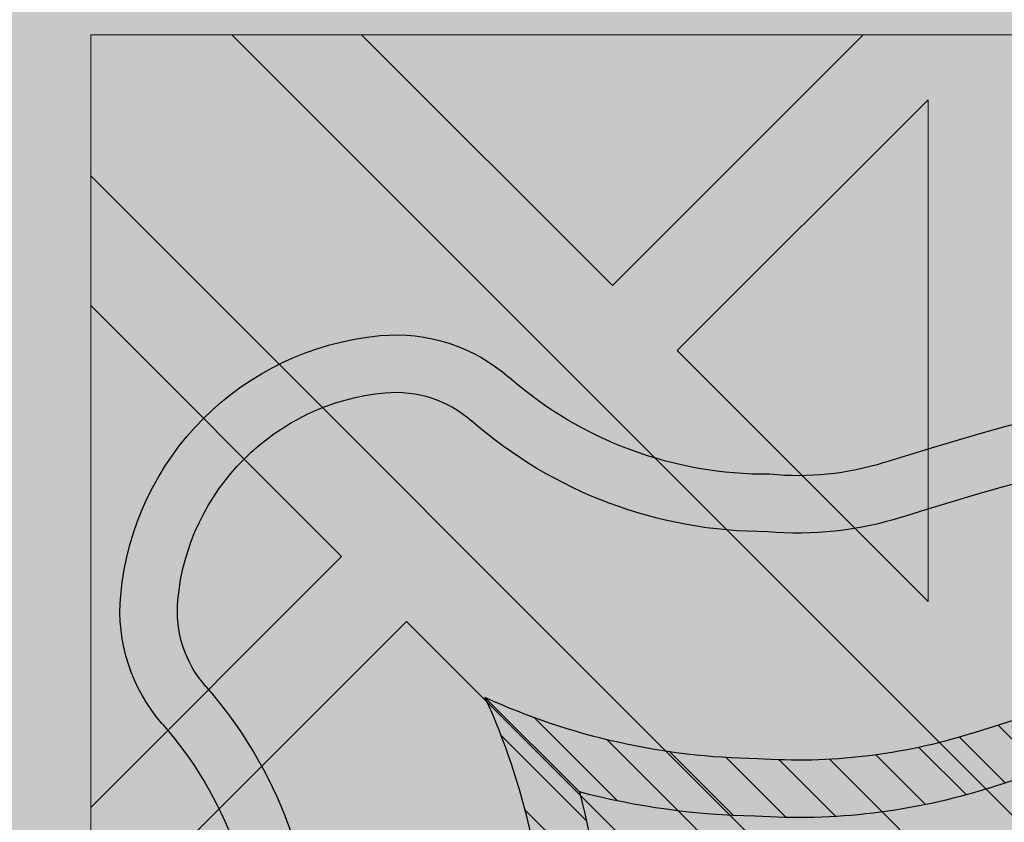
# Model space of a CAD drawing. Units: inches. Extents: x 844 to 2234, y 346 to 1084.
# Tile 81 of 93: x 1999.197 to 2001.933, y 708.742 to 710.971. Entities that reach past the tile are written whole.
import ezdxf

# ---------------------------------------------------------------- set-up
doc = ezdxf.new("R2010")
doc.units = ezdxf.units.IN
doc.header["$MEASUREMENT"] = 0
for name, color, linetype, lineweight in [('A-ANNO-DIMS', 2, 'Continuous', 18), ('furniture', 8, 'Continuous', 18), ('RA-AP-01$0$INT', 35, 'Continuous', 5)]:
    doc.layers.add(name, color=color, linetype=linetype, lineweight=lineweight)
doc.layers.add('RA-AP-01$0$FURN', color=3, linetype='Continuous')
doc.layers.add('RA-AP-01$0$WOOD', color=64, linetype='Continuous')
doc.styles.get("Standard").update_dxf_attribs({"font": 'arial.ttf'})
doc.dimstyles.get("Standard").update_dxf_attribs({"dimtxt": 6, "dimasz": 3, "dimexe": 0.18, "dimexo": 0.0625, "dimgap": 0.09, "dimtad": 0, "dimtih": 1, "dimtoh": 1, "dimdec": 1, "dimzin": 0, "dimdsep": 46, "dimlunit": 3, "dimtxsty": 'Standard', "dimblk": 'ARCHTICK', "dimcen": 0.09, "dimadec": 0, "dimazin": 0, "dimtfac": 1, "dimtdec": 1, "dimtofl": 0, "dimtmove": 0, "dimatfit": 3, "dimfxl": 1, "dimtolj": 1, "dimtzin": 0, "dimarcsym": 0})

# ---------------------------------------------------------------- blocks, each defined once
blk = doc.blocks.new('A$C18D01794')
at = {"layer": 'RA-AP-01$0$INT'}
blk.add_hatch(color=256, dxfattribs=at).paths.add_polyline_path([(4.505206456958071, -7.906712009588039), (5.305206456958072, -7.906712009588039), (5.305206456958072, -7.106712009588038), (5.255206456951893, -7.106712009588036), (5.25520645694868, -7.856712009570104), (4.555206456959269, -7.856712009588616), (4.555206456956052, -7.106712009588038), (4.505206456958073, -7.106712009588038)])
h = blk.add_hatch(color=256, dxfattribs=at)
h.paths.add_polyline_path([(4.585917135068448, -7.856712009587804), (4.614201406330596, -7.856712009587056), (4.668846067270487, -7.802067348644738), (4.723490728212344, -7.856712009584164), (4.771774999457151, -7.856712009582887), (4.826419660396886, -7.80206734864072), (4.862780050090322, -7.838427738332541), (4.844495778842715, -7.856712009580965), (4.862780050090411, -7.856712009580482), (4.905206456960182, -7.814285602707865), (4.947632863832445, -7.856712009578238), (4.965917135079675, -7.856712009577755), (4.947632863831759, -7.838427738330656), (4.983993253523576, -7.802067348637219), (5.038637914464627, -7.856712009575829), (5.08692218571208, -7.856712009574554), (5.141566846649976, -7.802067348634224), (5.196211507589851, -7.856712009571666), (5.224495778822615, -7.856712009570916), (4.905206456953975, -7.537422687702283)])
h.paths.add_polyline_path([(4.895206456956031, -7.575706958950402), (4.895206456958921, -7.684996280828174), (4.840561796018589, -7.630351619890275)], flags=16)
h.paths.add_polyline_path([(4.915206456955638, -7.575706958949956), (4.969851117895509, -7.630351619887399), (4.915206456957609, -7.684996280827732)], flags=16)
h.paths.add_polyline_path([(4.826419660395175, -7.644493755514321), (4.881064321335613, -7.699138416452331), (4.771774999456703, -7.69913841645522)], flags=16)
h.paths.add_polyline_path([(4.983993253519558, -7.644493755510815), (5.038637914460456, -7.699138416449285), (4.929348592581548, -7.69913841645126)], flags=16)
h.paths.add_polyline_path([(4.881064321336025, -7.719138416452334), (4.826419660397532, -7.773783077393256), (4.771774999457062, -7.719138416455217)], flags=16)
h.paths.add_polyline_path([(4.929348592582019, -7.71913841645126), (5.038637914460982, -7.719138416449284), (4.983993253522945, -7.773783077389749)], flags=16)
h.paths.add_polyline_path([(4.895206456960191, -7.733280552075633), (4.895206456962115, -7.806001331460164), (4.876922185715016, -7.824285602708492), (4.840561796021581, -7.787925213016675)], flags=16)
h.paths.add_polyline_path([(4.915206456958487, -7.733280552075187), (4.969851117899527, -7.787925213013798), (4.933490728206909, -7.824285602708034), (4.9152064569598, -7.806001331461736)], flags=16)
h.paths.add_polyline_path([(4.757632863832376, -7.733280552079264), (4.812277524772842, -7.787925213017304), (4.757632863834348, -7.842569873958233)], flags=16)
h.paths.add_polyline_path([(4.737632863832376, -7.73328055207979), (4.737632863834348, -7.842569873958701), (4.682988202893906, -7.787925213020692)], flags=16)
h.paths.add_polyline_path([(5.05278005008503, -7.733280552072701), (5.052780050087917, -7.842569873951664), (4.998135389146995, -7.787925213013169)], flags=16)
h.paths.add_polyline_path([(5.072780050085024, -7.733280552072333), (5.127424711025931, -7.787925213010806), (5.072780050087916, -7.842569873951244)], flags=16)
h.paths.add_polyline_path([(4.935917135072783, -7.506712009583784), (5.255206456948811, -7.826001331459767), (5.255206456948932, -7.797717060211899), (5.200561796010279, -7.743072399273238), (5.255206456949403, -7.688427738334128), (5.25520645694961, -7.640143467086677), (5.200561796009787, -7.585498806146837), (5.236922185702417, -7.549138416454212), (5.255206456949919, -7.56742268770172), (5.255206456949998, -7.549138416454178), (5.212780050078687, -7.506712009583814), (5.25520645695036, -7.464285602712145), (5.255206456950438, -7.446001331464763), (5.236922185702424, -7.464285602712779), (5.200561796009796, -7.427925213020149), (5.255206456950753, -7.373280552079203), (5.25520645695096, -7.324996280834394), (5.200561796010322, -7.270351619893748), (5.255206456951428, -7.215706958952649), (5.255206456951547, -7.187422687705071)])
h.paths.add_polyline_path([(5.042988202883395, -7.42792521302065), (5.097632863823085, -7.373280552080975), (5.097632863822622, -7.482569873959883)], flags=16)
h.paths.add_polyline_path([(5.028846067259663, -7.442067348644384), (5.083490728198774, -7.496712009583504), (4.974201406321001, -7.496712009583035)], flags=16)
h.paths.add_polyline_path([(5.117632863823087, -7.37328055208089), (5.172277524762331, -7.42792521302015), (5.11763286382262, -7.482569873959851)], flags=16)
h.paths.add_polyline_path([(5.08349072819877, -7.516712009582191), (5.028846067259652, -7.571356670521302), (4.974201406320998, -7.516712009582638)], flags=16)
h.paths.add_polyline_path([(5.131774999446817, -7.35913841645716), (5.186419660386065, -7.413783077396415), (5.241064321325782, -7.359138416456712)], flags=17)
h.paths.add_polyline_path([(5.131774999446228, -7.496712009583703), (5.186419660386065, -7.442067348643883), (5.222780050079488, -7.478427738337313), (5.204495778832781, -7.496712009584014)], flags=16)
h.paths.add_polyline_path([(5.097632863822613, -7.530854145205813), (5.097632863823061, -7.640143467084723), (5.042988202883383, -7.585498806145032)], flags=16)
h.paths.add_polyline_path([(5.131774999446899, -7.339138416457162), (5.241064321325809, -7.339138416456712), (5.186419660386591, -7.284493755517479)], flags=17)
h.paths.add_polyline_path([(5.131774999446226, -7.516712009581999), (5.204495778830767, -7.516712009581702), (5.22278005007868, -7.534996280829206), (5.186419660386049, -7.571356670521828)], flags=16)
h.paths.add_polyline_path([(5.11763286382262, -7.530854145205852), (5.17227752476232, -7.585498806145562), (5.117632863823064, -7.64014346708481)], flags=16)
h.paths.add_polyline_path([(5.186419660386069, -7.599640941770585), (5.241064321325754, -7.654285602710281), (5.131774999446791, -7.654285602709814)], flags=16)
h.paths.add_polyline_path([(5.131774999446872, -7.674285602709813), (5.24106432132578, -7.674285602710282), (5.186419660386554, -7.728930263649504)], flags=16)
h.paths.add_polyline_path([(5.255206456951811, -7.126001331467467), (5.255206456951895, -7.106712009588038), (4.555206456956052, -7.106712009588038), (4.555206456956136, -7.12600133146746), (4.905206456953973, -7.476001331465289)])
h.paths.add_polyline_path([(4.983993253513404, -7.368930263651977), (4.92934859257295, -7.314285602713969), (5.03863791445186, -7.314285602711063)], flags=16)
h.paths.add_polyline_path([(4.969851117889988, -7.383072399276016), (4.915206456952556, -7.437717060215906), (4.915206456949648, -7.328427738338133)], flags=16)
h.paths.add_polyline_path([(4.929348592572535, -7.294285602713971), (4.983993253511019, -7.239640941773039), (5.038637914451496, -7.294285602711065)], flags=16)
h.paths.add_polyline_path([(5.052780050074912, -7.280143467087016), (4.998135389134438, -7.225498806148989), (5.052780050072919, -7.170854145208052)], flags=16)
h.paths.add_polyline_path([(5.07278005007491, -7.280143467086489), (5.072780050072918, -7.170854145207579), (5.127424711013374, -7.225498806145578)], flags=16)
h.paths.add_polyline_path([(4.89520645695295, -7.437717060216355), (4.840561796013067, -7.383072399278919), (4.895206456950961, -7.328427738338582)], flags=16)
h.paths.add_polyline_path([(4.915206456948365, -7.280143467090674), (4.915206456946434, -7.207422687704125), (4.933490728192729, -7.18913841645701), (4.969851117886972, -7.225498806149623)], flags=16)
h.paths.add_polyline_path([(4.881064321327021, -7.314285602715054), (4.82641966038902, -7.368930263655506), (4.771774999448108, -7.314285602717047)], flags=16)
h.paths.add_polyline_path([(4.895206456950073, -7.280143467091125), (4.840561796009022, -7.225498806152518), (4.876922185700835, -7.18913841645908), (4.895206456948749, -7.207422687706589)], flags=16)
h.paths.add_polyline_path([(4.983993253510392, -7.211356670525576), (4.947632863816944, -7.174996280833758), (4.965917135064043, -7.156712009585847), (5.038637914448995, -7.156712009584522)], flags=16)
h.paths.add_polyline_path([(4.881064321326543, -7.294285602715056), (4.771774999447578, -7.294285602717046), (4.826419660385607, -7.239640941776569)], flags=16)
h.paths.add_polyline_path([(4.905206456946447, -7.19913841645844), (4.862780050074785, -7.156712009587725), (4.947632863816685, -7.156712009586302)], flags=16)
h.paths.add_polyline_path([(5.14156684663679, -7.211356670521528), (5.086922185696452, -7.156712009583639), (5.196211507574223, -7.156712009581651)], flags=16)
h.paths.add_polyline_path([(4.8264196603837, -7.211356670529104), (4.771774999442643, -7.156712009590501), (4.8444957788276, -7.156712009588568), (4.862780050075511, -7.17499628083566)], flags=16)
h.paths.add_polyline_path([(4.812277524760289, -7.225498806153156), (4.757632863822258, -7.28014346709363), (4.757632863819352, -7.170854145214669)], flags=16)
h.paths.add_polyline_path([(4.73763286382226, -7.280143467093997), (4.682988202881349, -7.22549880615554), (4.737632863819352, -7.170854145215086)], flags=16)
h.paths.add_polyline_path([(4.723490728195188, -7.156712009591787), (4.668846067257299, -7.211356670532127), (4.614201406317417, -7.156712009594693)], flags=16)
h.paths.add_polyline_path([(4.597632863829262, -7.506712009583814), (4.555206456957951, -7.54913841645418), (4.555206456958029, -7.56742268770172), (4.573490728205535, -7.549138416454212), (4.609851117898167, -7.585498806146839), (4.555206456958338, -7.640143467086675), (4.555206456958546, -7.688427738334125), (4.60985111789767, -7.743072399273238), (4.555206456959015, -7.797717060211899), (4.555206456959138, -7.826001331459767), (4.874495778835167, -7.506712009583786), (4.5552064569564, -7.187422687705062), (4.555206456956523, -7.215706958952644), (4.609851117897629, -7.270351619893746), (4.555206456956988, -7.324996280834396), (4.555206456957198, -7.373280552079195), (4.609851117898153, -7.427925213020147), (4.573490728205528, -7.464285602712779), (4.555206456957507, -7.446001331464756), (4.555206456957585, -7.464285602712143)])
h.paths.add_polyline_path([(4.712780050085332, -7.482569873959882), (4.712780050084863, -7.373280552080972), (4.767424711024555, -7.42792521302065)], flags=16)
h.paths.add_polyline_path([(4.726922185709173, -7.496712009583504), (4.781566846648288, -7.442067348644384), (4.836211507586949, -7.496712009583033)], flags=16)
h.paths.add_polyline_path([(4.692780050085327, -7.482569873959851), (4.638135389145619, -7.427925213020149), (4.692780050084865, -7.373280552080892)], flags=16)
h.paths.add_polyline_path([(4.726922185709182, -7.516712009582191), (4.836211507586949, -7.51671200958264), (4.7815668466483, -7.571356670521304)], flags=16)
h.paths.add_polyline_path([(4.678637914461726, -7.496712009583706), (4.605917135075169, -7.496712009584014), (4.587632863828464, -7.478427738337311), (4.623993253521887, -7.442067348643881)], flags=16)
h.paths.add_polyline_path([(4.712780050085336, -7.530854145205816), (4.767424711024568, -7.585498806145034), (4.71278005008489, -7.640143467084724)], flags=16)
h.paths.add_polyline_path([(4.678637914461726, -7.516712009582001), (4.623993253521899, -7.571356670521829), (4.587632863829271, -7.534996280829206), (4.605917135077185, -7.5167120095817)], flags=16)
h.paths.add_polyline_path([(4.692780050085336, -7.530854145205848), (4.692780050084889, -7.64014346708481), (4.638135389145632, -7.585498806145562)], flags=16)
h.paths.add_polyline_path([(4.623993253521885, -7.413783077396415), (4.678637914461131, -7.359138416457161), (4.56934859258217, -7.359138416456712)], flags=17)
h.paths.add_polyline_path([(4.623993253521901, -7.599640941770568), (4.678637914461158, -7.654285602709814), (4.569348592582195, -7.654285602710281)], flags=16)
h.paths.add_polyline_path([(4.678637914461051, -7.339138416457162), (4.623993253521361, -7.284493755517479), (4.569348592582143, -7.339138416456712)], flags=17)
h.paths.add_polyline_path([(4.678637914461076, -7.674285602709813), (4.623993253521399, -7.728930263649504), (4.569348592582167, -7.674285602710281)], flags=16)
h = blk.add_hatch(color=256, dxfattribs=at)
h.paths.add_polyline_path([(4.905206456954232, -7.537422687702028), (4.874495778835232, -7.506712009583718), (4.555206456959138, -7.826001331459766), (4.555206456959269, -7.856712009588616), (4.585917135068449, -7.856712009587804)])
h.paths.add_polyline_path([(4.935917135072152, -7.506712009583152), (4.905206456953497, -7.537422687701806), (5.224495778822614, -7.856712009570917), (5.255206456948681, -7.856712009570104), (5.255206456948813, -7.826001331459768)])
h.paths.add_polyline_path([(5.255206456951549, -7.18742268770507), (5.255206456951813, -7.126001331467461), (4.905206456953563, -7.476001331465701), (4.935917135072559, -7.506712009584006)])
h.paths.add_polyline_path([(4.874495778835167, -7.506712009583785), (4.905206456953818, -7.476001331465132), (4.555206456956135, -7.126001331467458), (4.555206456956399, -7.187422687705064)])
h = blk.add_hatch(color=256, dxfattribs=at)
h.paths.add_polyline_path([(5.028846067259997, -7.571356670520955), (4.974201406321342, -7.516712009582294), (5.083490728199115, -7.516712009581846)])
h.paths.add_polyline_path([(4.974201406321344, -7.496712009582688), (5.028846067260004, -7.442067348644037), (5.083490728199117, -7.496712009583157)])
h.paths.add_polyline_path([(5.042988202883738, -7.427925213020309), (5.097632863823428, -7.373280552080627), (5.097632863822963, -7.482569873959537)])
h.paths.add_polyline_path([(5.117632863822961, -7.482569873959509), (5.117632863823428, -7.373280552080546), (5.172277524762674, -7.427925213019804)])
h.paths.add_polyline_path([(5.131774999446572, -7.496712009583358), (5.186419660386406, -7.442067348643536), (5.222780050079831, -7.478427738336961), (5.204495778833122, -7.496712009583667)])
h.paths.add_polyline_path([(5.236922185702764, -7.464285602712433), (5.200561796010139, -7.427925213019802), (5.255206456949971, -7.373280552079975), (5.255206456950271, -7.446001331464927)])
h.paths.add_polyline_path([(5.186419660386412, -7.41378307739607), (5.131774999447164, -7.359138416456815), (5.241064321326123, -7.359138416456366)])
h.paths.add_polyline_path([(5.131774999447238, -7.339138416456815), (5.186419660386934, -7.284493755517132), (5.241064321326153, -7.339138416456368)])
h.paths.add_polyline_path([(5.200561796010663, -7.270351619893402), (5.255206456949324, -7.215706958954747), (5.255206456949777, -7.324996280832518)])
h.paths.add_polyline_path([(5.21278005007903, -7.50671200958347), (5.255206456950223, -7.464285602712278), (5.255206456950696, -7.549138416454185)])
h.paths.add_polyline_path([(5.13177499944657, -7.516712009581652), (5.204495778831106, -7.516712009581354), (5.222780050079024, -7.534996280828858), (5.186419660386397, -7.571356670521485)])
h.paths.add_polyline_path([(5.117632863823405, -7.640143467084465), (5.117632863822955, -7.530854145205498), (5.172277524762665, -7.585498806145217)])
h.paths.add_polyline_path([(5.042988202883727, -7.585498806144689), (5.097632863822957, -7.530854145205474), (5.097632863823407, -7.64014346708438)])
h.paths.add_polyline_path([(5.131774999447135, -7.654285602709467), (5.186419660386394, -7.599640941770219), (5.241064321326097, -7.654285602709933)])
h.paths.add_polyline_path([(5.200561796010128, -7.585498806146492), (5.236922185702758, -7.549138416453866), (5.255206456950264, -7.567422687701371), (5.255206456949948, -7.640143467086325)])
h.paths.add_polyline_path([(5.186419660386895, -7.728930263649157), (5.131774999447213, -7.674285602709467), (5.241064321326127, -7.674285602709934)])
h.paths.add_polyline_path([(5.200561796010624, -7.743072399272893), (5.255206456949745, -7.688427738333778), (5.255206456949276, -7.797717060211553)])
h = blk.add_hatch(color=256, dxfattribs=at)
h.paths.add_polyline_path([(4.969851117891331, -7.630351619889621), (4.915206456952669, -7.575706958950966), (4.915206456952222, -7.684996280828739)])
h.paths.add_polyline_path([(4.895206456953064, -7.575706958950968), (4.840561796014413, -7.630351619889628), (4.895206456953533, -7.684996280828741)])
h.paths.add_polyline_path([(4.826419660390684, -7.644493755513362), (4.771774999451003, -7.699138416453052), (4.881064321329913, -7.699138416452587)])
h.paths.add_polyline_path([(4.881064321329884, -7.719138416452585), (4.771774999450921, -7.719138416453052), (4.82641966039018, -7.773783077392298)])
h.paths.add_polyline_path([(4.895206456953734, -7.733280552076196), (4.840561796013912, -7.787925213016031), (4.876922185707337, -7.824285602709455), (4.895206456954043, -7.806001331462747)])
h.paths.add_polyline_path([(4.862780050082808, -7.838427738332388), (4.826419660390178, -7.802067348639763), (4.771774999450351, -7.856712009579595), (4.844495778835303, -7.856712009579895)])
h.paths.add_polyline_path([(4.812277524766446, -7.787925213016036), (4.757632863827191, -7.733280552076788), (4.757632863826741, -7.842569873955747)])
h.paths.add_polyline_path([(4.737632863827191, -7.733280552076863), (4.682988202887508, -7.787925213016558), (4.737632863826743, -7.842569873955778)])
h.paths.add_polyline_path([(4.668846067263777, -7.802067348640287), (4.614201406325123, -7.856712009578949), (4.723490728202894, -7.856712009579402)])
h.paths.add_polyline_path([(4.905206456953846, -7.814285602708654), (4.862780050082654, -7.856712009579847), (4.947632863824561, -7.85671200958032)])
h.paths.add_polyline_path([(4.915206456952028, -7.733280552076195), (4.91520645695173, -7.806001331460731), (4.933490728199234, -7.824285602708648), (4.96985111789186, -7.787925213016022)])
h.paths.add_polyline_path([(5.038637914454841, -7.719138416453029), (4.929348592575874, -7.71913841645258), (4.983993253515593, -7.773783077392289)])
h.paths.add_polyline_path([(4.983993253515065, -7.644493755513352), (4.929348592575849, -7.699138416452582), (5.038637914454755, -7.699138416453031)])
h.paths.add_polyline_path([(5.052780050079843, -7.73328055207676), (4.998135389140595, -7.787925213016018), (5.052780050080309, -7.842569873955721)])
h.paths.add_polyline_path([(4.983993253516868, -7.802067348639752), (4.947632863824241, -7.838427738332383), (4.965917135071747, -7.856712009579888), (5.038637914456701, -7.856712009579572)])
h.paths.add_polyline_path([(5.127424711019533, -7.787925213016519), (5.072780050079843, -7.733280552076838), (5.07278005008031, -7.842569873955751)])
h.paths.add_polyline_path([(5.141566846643269, -7.802067348640248), (5.086922185704154, -7.85671200957937), (5.196211507581929, -7.856712009578901)])
for p, q in [((5.255206456951895, -7.106712009588038), (5.255206456948681, -7.856712009570104)), ((4.935917135072783, -7.506712009583784), (5.255206456948813, -7.826001331459769)), ((4.905206456953975, -7.537422687702283), (5.224495778822613, -7.856712009570916)), ((5.18641966038655, -7.728930263649502), (5.131774999446872, -7.674285602709813)), ((5.241064321325782, -7.674285602710281), (5.186419660386552, -7.728930263649504)), ((5.255206456949399, -7.68842773833413), (5.200561796010281, -7.743072399273238)), ((5.12742471102593, -7.787925213010804), (5.072780050085028, -7.733280552072336)), ((5.072780050085028, -7.733280552072336), (5.072780050087916, -7.842569873951246)), ((5.255206456948934, -7.797717060211899), (5.200561796010281, -7.743072399273238)), ((5.072780050087916, -7.842569873951246), (5.127424711025931, -7.787925213010806)), ((5.086922185712082, -7.85671200957455), (5.141566846649976, -7.802067348634222)), ((5.196211507589851, -7.856712009571664), (5.141566846649976, -7.802067348634222)), ((4.555206456959269, -7.856712009588616), (5.255206456948681, -7.856712009570104))]:
    blk.add_line(p, q, dxfattribs=at)
blk = doc.blocks.new('A$C32926AE1')
at = {"layer": 'RA-AP-01$0$WOOD'}
h = blk.add_hatch(color=256, dxfattribs=at)
h.dxf.hatch_style = 1
h.paths.add_polyline_path([(5.157430609644524, 4.573483066760929, -0.1009492694046607), (5.155401577623758, 4.593365984175333, -0.1842662638101597), (5.172249623284174, 4.638795604568598, 0.2056608120311276), (5.179560981299304, 4.661316324430096, 0.3614336704623542), (5.134352340494423, 4.706524965234944, 0.2056608120311297), (5.111831620632933, 4.699213607219793, -0.1842662638101113), (5.066402000239693, 4.682365561559342, -0.1055311479399994), (5.045656153913092, 4.68467289944697, 0.1567636581983829), (4.763886414745334, 4.684672899446966, -0.1055311479399895), (4.743140568418733, 4.68236556155934, -0.1842662638100833), (4.6977109480255, 4.69921360721979, 0.2056608120302612), (4.675190228164109, 4.706524965234949, 0.3614336704708441), (4.629981587358889, 4.66131632442871, 0.2056608120245944), (4.637292945374126, 4.638795604567974, -0.1842662638101024), (4.654140991034615, 4.59336598417475, -0.1009492694055169), (4.652111959013835, 4.573483066760181, 0.021410119221476), (4.629748025606143, 4.156712009541676, 0.0214101192214795), (4.652111959013809, 3.739940952323101, -0.1009492694059586), (4.654140991034615, 3.720058034908448, -0.1842662638100975), (4.637292945374126, 3.674628414515226, 0.2056608120245705), (4.629981587358889, 3.652107694654492, 0.3614336704708879), (4.675190228164113, 3.606899053848249, 0.2056608120302384), (4.697710948025501, 3.614210411863408, -0.1842662638100995), (4.743140568418738, 3.63105845752386, -0.1055311479402541), (4.763886414745388, 3.628751119636215, 0.1567636581983776), (5.045656153913137, 3.628751119636244, -0.1055311479397538), (5.066402000239692, 3.631058457523857, -0.1842662638101067), (5.111831620632931, 3.614210411863407, 0.2056608120310924), (5.134352340494417, 3.606899053848256, 0.3614336704624001), (5.179560981299307, 3.652107694653103, 0.2056608120311314), (5.172249623284175, 3.6746284145146, -0.1842662638101402), (5.155401577623758, 3.72005803490786, -0.1009492694051366), (5.15743060964455, 3.739940952322354, 0.0214101192215073), (5.179794543052287, 4.156712009541468, 0.0214101192215252)])
h.paths.add_polyline_path([(4.639748609479751, 4.156712009541513, 0.0213537860821624), (4.661970494867118, 3.741887061152232, -0.094075836301374), (4.664143710413708, 3.7196126951003, -0.1824818158568985), (4.644813765429836, 3.668037719127816, 0.2056608120245319), (4.639939526753007, 3.653023905887301, 0.3614336704710246), (4.676106439397173, 3.616856993242342, 0.2056608120302234), (4.691120252638095, 3.621731231919122, -0.1824818158602558), (4.742695228611606, 3.641061176902986, -0.1029891339458722), (4.766991894714349, 3.638256818950944, 0.156709409989566), (5.042550673941472, 3.638256818950105, -0.102989133958497), (5.066847340047078, 3.641061176902949, -0.1824818158594995), (5.118422316020358, 3.621731231919103, 0.2056608120311416), (5.133436129261316, 3.616856993242346, 0.3614336704621468), (5.169603041905217, 3.653023905886178, 0.2056608120310986), (5.164728803228477, 3.668037719127177, -0.1824818158565612), (5.145398858244737, 3.719612695099578, -0.0940758363009313), (5.147572073791232, 3.741887061151398, 0.0213537860822023), (5.169793959178681, 4.156712009541451, 0.0213537860822226), (5.147572073791203, 4.571536957931898, -0.0940758363005034), (5.145398858244737, 4.59381132398362, -0.1824818158565587), (5.164728803228476, 4.645386299956021, 0.2056608120311045), (5.169603041905216, 4.66040011319702, 0.3614336704621845), (5.133436129261313, 4.696567025840856, 0.2056608120310773), (5.118422316020359, 4.691692787164098, -0.182481815859508), (5.066847340047078, 4.67236284218025, -0.1029891339584606), (5.04255067394148, 4.675167200133092, 0.156709409989566), (4.766991894714357, 4.675167200132257, -0.1029891339458842), (4.742695228611611, 4.672362842180213, -0.1824818158602725), (4.691120252638095, 4.691692787164077, 0.2056608120302152), (4.676106439397174, 4.696567025840858, 0.3614336704710363), (4.639939526753005, 4.660400113195899, 0.2056608120245495), (4.644813765429837, 4.645386299955384, -0.1824818158568934), (4.664143710413708, 4.593811323982902, -0.0940758363009187), (4.661970494867149, 4.571536957931074, 0.021353786082177)], flags=16)
h.paths.add_polyline_path([(5.129794543052235, 4.432167055276933, -0.0141661062790638), (5.130152669293814, 4.156927903047693, -0.0141661062790647), (5.129794543052234, 3.881688750818433, -0.0785247771143638), (5.10979738006795, 3.755143611847103, 0.0945969212073497), (5.105408519571111, 3.717898134952927, 0.1043170707844957), (5.116074640131521, 3.670385395016088, 0.1043170707864965), (5.068561900193738, 3.681051515576561, 0.09459692119553), (5.031316423304057, 3.676662655080835, -0.1580239521427272), (4.778226145355827, 3.676662655080367, 0.0945969211986668), (4.740980668464973, 3.681051515576592, 0.1043170707882822), (4.693467928526415, 3.670385395015844, 0.1043170707867916), (4.704134049087309, 3.717898134953662, 0.0945969211972894), (4.69974518859162, 3.755143611844042, -0.0785247771163196), (4.679748025606343, 3.881688750818406, -0.0141661062790663), (4.679389899364763, 4.156927903047693, -0.0141661062790672), (4.679748025606343, 4.432167055276998, -0.0785247771163064), (4.699745188591625, 4.55871219425134, 0.094596921197333), (4.704134049087308, 4.595957671141738, 0.1043170707867205), (4.693467928526416, 4.643470411079523, 0.1043170707882628), (4.740980668464965, 4.632804290518776, 0.0945969211988114), (4.778226145355874, 4.637193151015016, -0.158023952142669), (5.031316423304015, 4.637193151014546, 0.0945969211956361), (5.068561900193736, 4.632804290518806, 0.1043170707864979), (5.11607464013152, 4.643470411079278, 0.1043170707844617), (5.105408519571112, 4.595957671142455, 0.0945969212074597), (5.109797380067959, 4.558712194248236, -0.0785247771143467)], flags=0)
h.paths.add_polyline_path([(5.119794532311105, 4.432259799204851, -0.0142000800617244), (5.120156169157484, 4.156927903047701, -0.0142000800617277), (5.119794532311105, 3.881596006890482, -0.0784894509520253), (5.100273383573699, 3.758192358677797, 0.0940138827242913), (5.095413455884425, 3.717477693979438, 0.0606271852308753), (5.099615656341024, 3.686844378806616, 0.0606271852322524), (5.068982341167493, 3.691046579263239, 0.0940138827010453), (5.028267676478798, 3.686186651576848, -0.1580706864508061), (4.781274892180912, 3.686186651576435, 0.0940138827026903), (4.740560227491556, 3.691046579263279, 0.0606271852339895), (4.709926912317155, 3.686844378806508, 0.0606271852329405), (4.714129112773991, 3.717477693980356, 0.094013882701304), (4.709269185087677, 3.758192358669163, -0.0784894509577193), (4.689748036347473, 3.881596006890469, -0.014200080061729), (4.689386399501094, 4.156927903047709, -0.0142000800617217), (4.689748036347473, 4.432259799204808, -0.078489450957724), (4.709269185087651, 4.555663447426125, 0.0940138827014585), (4.714129112773992, 4.596378112114996, 0.0606271852329731), (4.709926912317154, 4.62701142728886, 0.0606271852340196), (4.74056022749157, 4.622809226832087, 0.0940138827024997), (4.781274892180847, 4.627669154518912, -0.1580706864508359), (5.028267676478777, 4.627669154518526, 0.0940138827010946), (5.068982341167492, 4.622809226832129, 0.060627185232254), (5.099615656341024, 4.627011427288751, 0.0606271852308727), (5.095413455884425, 4.59637811211593, 0.0940138827241088), (5.100273383573675, 4.555663447417647, -0.0784894509520978)], flags=0)
h.paths.add_polyline_path([(5.06978912287499, 4.430218106756144, -0.014241683694547), (5.070173729147532, 4.156927903047672, -0.0142416836945458), (5.06978912287499, 3.883637699339223, -0.0800609523125196), (5.052662118612511, 3.773463122773442, 0.0526421978001116), (5.04590916754064, 3.740550867606997, 0.0526421977992423), (5.012996912374707, 3.73379791653534, -0.1583028414718258), (4.796545656286308, 3.73379791653451, 0.0526421978034211), (4.763633401117837, 3.740550867607021, 0.0526421978018622), (4.756880450045755, 3.773463122774558, -0.0800609523117106), (4.739753445783639, 3.883637699339268, -0.0142416836945435), (4.739368839511098, 4.156927903047671, -0.0142416836945477), (4.739753445783639, 4.430218106756155, -0.0800609523116345), (4.75688045004574, 4.540392683320762, 0.052642197801941), (4.763633401117837, 4.573304938488346, 0.0526421978035071), (4.796545656286361, 4.580057889560873, -0.1583028414717561), (5.012996912374669, 4.580057889560039, 0.0526421977993048), (5.04590916754064, 4.57330493848837, 0.0526421978002057), (5.052662118612529, 4.540392683321868, -0.080060952312477)], flags=0)
h.paths.add_polyline_path([(5.049789715110557, 4.43038092723357, -0.0143097550741839), (5.05018085590259, 4.156927903047715, -0.0143097550741854), (5.049789715110558, 3.883474878861827, -0.0800685599149176), (5.03362098255317, 3.779581877367999, 0.0306258898956367), (5.028241146483733, 3.758218888663947, 0.0306258898977031), (5.006878157778253, 3.75283905259408, -0.1583983521624096), (4.802664410878162, 3.752839052594731, 0.0306258898946014), (4.781301422174808, 3.758218888663924, 0.0306258898967912), (4.775921586105202, 3.779581877368794, -0.080068559914251), (4.759752853548071, 3.883474878861786, -0.0143097550741854), (4.759361712756037, 4.156927903047671, -0.0143097550741854), (4.759752853548071, 4.430380927233557, -0.0800685599142479), (4.775921586105193, 4.534273928726546, 0.0306258898968306), (4.781301422174808, 4.555636917431444, 0.0306258898945754), (4.802664410878143, 4.561016753500631, -0.1583983521624168), (5.006878157778244, 4.561016753501291, 0.0306258898977177), (5.028241146483733, 4.555636917431421, 0.0306258898958182), (5.03362098255321, 4.534273928727244, -0.080068559914796)], flags=0)
h.paths.add_polyline_path([(4.999766070382627, 4.428171244713864, -0.0143443147609634), (5.000198441819402, 4.156927903047689, -0.0143443147609612), (4.999766070382627, 3.885684561381556, -0.0784641635803329), (4.987356730658798, 3.799103304488872, -0.1506053783831347), (4.822185837999821, 3.79910330448882, -0.0784641635803318), (4.809776498276007, 3.885684561381509, -0.014344314760963), (4.809344126839227, 4.156927903047677, -0.0143443147609645), (4.809776498276007, 4.428171244713873, -0.0784641635803192), (4.822185837999822, 4.514752501606549, -0.1506053783831338), (4.987356730658798, 4.514752501606494, -0.078464163580285)], flags=0)
h.paths.add_polyline_path([(4.979755254238824, 4.42764379880488, -0.0143772539198268), (4.980205517789977, 4.156927903047693, -0.0143772539198275), (4.979755254238824, 3.886212007290489, -0.0689242507424422), (4.971183264704897, 3.815276770442801, -0.1296645318904179), (4.838359303953726, 3.815276770442746, -0.0689242507424186), (4.829787314419809, 3.886212007290419, -0.0143772539198292), (4.829337050868653, 4.156927903047653, -0.0143772539198325), (4.829787314419809, 4.427643798804946, -0.0689242507424211), (4.838359303953725, 4.498579035652621, -0.1296645318904187), (4.971183264704897, 4.498579035652565, -0.0689242507424401)], flags=0)
h = blk.add_hatch(color=256, dxfattribs=at)
h.dxf.hatch_style = 1
h.paths.add_polyline_path([(5.145398858244737, 4.59381132398362, -0.1824818158565616), (5.164728803228476, 4.645386299956021, 0.2056608120311045), (5.169603041905216, 4.66040011319702, 0.3614336704621845), (5.133436129261313, 4.696567025840856, 0.2056608120310773), (5.118422316020359, 4.691692787164098, -0.182481815859508), (5.066847340047078, 4.67236284218025, -0.1029891339584606), (5.04255067394148, 4.675167200133092, 0.156709409989566), (4.766991894714357, 4.675167200132257, -0.1029891339458842), (4.742695228611611, 4.672362842180213, -0.1824818158602725), (4.691120252638095, 4.691692787164077, 0.2056608120302152), (4.676106439397174, 4.696567025840858, 0.3614336704710363), (4.639939526753005, 4.660400113195899, 0.2056608120245495), (4.644813765429837, 4.645386299955384, -0.1824818158568934), (4.664143710413708, 4.593811323982902, -0.0940758363009187), (4.661970494867149, 4.571536957931074, 0.0213537860821772), (4.639748609479751, 4.156712009541507, 0.0213537860821625), (4.661970494867119, 3.741887061152226, -0.0940758363013071), (4.664143710413708, 3.719612695100309, -0.1824818158569294), (4.644813765429836, 3.668037719127816, 0.2056608120245319), (4.639939526753007, 3.653023905887301, 0.3614336704710246), (4.676106439397173, 3.616856993242342, 0.2056608120302234), (4.691120252638095, 3.621731231919122, -0.1824818158602558), (4.742695228611606, 3.641061176902986, -0.1029891339458722), (4.766991894714349, 3.638256818950944, 0.156709409989566), (5.042550673941472, 3.638256818950105, -0.102989133958497), (5.066847340047078, 3.641061176902949, -0.1824818158594995), (5.118422316020358, 3.621731231919103, 0.2056608120311416), (5.133436129261316, 3.616856993242346, 0.3614336704621468), (5.169603041905217, 3.653023905886178, 0.2056608120310986), (5.164728803228477, 3.668037719127177, -0.1824818158565612), (5.145398858244737, 3.719612695099578, -0.0940758363009313), (5.147572073791232, 3.741887061151398, 0.0213537860822023), (5.169793959178681, 4.156712009541451, 0.0213537860822226), (5.147572073791203, 4.571536957931898, -0.0940758363004996)])
h.paths.add_polyline_path([(5.109797380067958, 4.55871219424824, -0.0785247771143472), (5.129794543052234, 4.432167055276936, -0.0141661062790644), (5.130152669293814, 4.156927903047685, -0.014166106279066), (5.129794543052234, 3.881688750818401, -0.0785247771143517), (5.109797380067946, 3.755143611847092, 0.0945969212073132), (5.105408519571111, 3.717898134952929, 0.1043170707844995), (5.116074640131521, 3.670385395016088, 0.1043170707864965), (5.068561900193738, 3.681051515576561, 0.09459692119553), (5.031316423304057, 3.676662655080835, -0.1580239521427272), (4.778226145355827, 3.676662655080367, 0.0945969211986668), (4.740980668464973, 3.681051515576592, 0.1043170707882822), (4.693467928526415, 3.670385395015844, 0.1043170707867916), (4.704134049087309, 3.717898134953662, 0.0945969211972894), (4.69974518859162, 3.755143611844042, -0.0785247771163196), (4.679748025606343, 3.881688750818406, -0.0141661062790663), (4.679389899364763, 4.156927903047693, -0.0141661062790672), (4.679748025606343, 4.432167055276998, -0.0785247771163064), (4.699745188591625, 4.55871219425134, 0.094596921197333), (4.704134049087308, 4.595957671141738, 0.1043170707867205), (4.693467928526416, 4.643470411079523, 0.1043170707882628), (4.740980668464965, 4.632804290518776, 0.0945969211988114), (4.778226145355874, 4.637193151015016, -0.158023952142669), (5.031316423304015, 4.637193151014546, 0.0945969211956361), (5.068561900193736, 4.632804290518806, 0.1043170707864979), (5.11607464013152, 4.643470411079278, 0.1043170707844617), (5.105408519571112, 4.595957671142455, 0.0945969212074504)], flags=16)
h.paths.add_polyline_path([(5.100273383573655, 4.55566344741771, -0.0784894509521388), (5.119794532311105, 4.432259799204852, -0.0142000800617252), (5.120156169157484, 4.156927903047686, -0.014200080061726), (5.119794532311105, 3.881596006890502, -0.0784894509520446), (5.100273383573696, 3.758192358677786, 0.0940138827242721), (5.095413455884425, 3.717477693979436, 0.0606271852308692), (5.099615656341024, 3.686844378806616, 0.0606271852322522), (5.068982341167493, 3.691046579263239, 0.0940138827010453), (5.028267676478798, 3.686186651576848, -0.1580706864508061), (4.781274892180912, 3.686186651576435, 0.0940138827026903), (4.740560227491556, 3.691046579263279, 0.0606271852339895), (4.709926912317155, 3.686844378806508, 0.0606271852329405), (4.714129112773991, 3.717477693980356, 0.094013882701304), (4.709269185087677, 3.758192358669163, -0.0784894509577193), (4.689748036347473, 3.881596006890469, -0.014200080061729), (4.689386399501094, 4.156927903047709, -0.0142000800617217), (4.689748036347473, 4.432259799204808, -0.078489450957724), (4.709269185087651, 4.555663447426125, 0.0940138827014585), (4.714129112773992, 4.596378112114996, 0.0606271852329731), (4.709926912317154, 4.62701142728886, 0.0606271852340196), (4.74056022749157, 4.622809226832087, 0.0940138827024997), (4.781274892180847, 4.627669154518912, -0.1580706864508359), (5.028267676478777, 4.627669154518526, 0.0940138827010946), (5.068982341167492, 4.622809226832129, 0.060627185232254), (5.099615656341024, 4.627011427288751, 0.0606271852308727), (5.095413455884425, 4.59637811211593, 0.094013882723957)], flags=0)
h.paths.add_polyline_path([(5.04590916754064, 4.57330493848837, 0.0526421978002057), (5.052662118612529, 4.540392683321868, -0.0800609523124783), (5.06978912287499, 4.430218106756142, -0.0142416836945469), (5.070173729147532, 4.156927903047672, -0.0142416836945458), (5.06978912287499, 3.883637699339223, -0.0800609523125196), (5.052662118612511, 3.773463122773442, 0.0526421978001116), (5.04590916754064, 3.740550867606997, 0.0526421977992423), (5.012996912374707, 3.73379791653534, -0.1583028414718258), (4.796545656286308, 3.73379791653451, 0.0526421978034211), (4.763633401117837, 3.740550867607021, 0.0526421978018622), (4.756880450045755, 3.773463122774558, -0.0800609523117106), (4.739753445783639, 3.883637699339268, -0.0142416836945435), (4.739368839511098, 4.156927903047671, -0.0142416836945477), (4.739753445783639, 4.430218106756155, -0.0800609523116345), (4.75688045004574, 4.540392683320762, 0.052642197801941), (4.763633401117837, 4.573304938488346, 0.0526421978035071), (4.796545656286361, 4.580057889560873, -0.1583028414717561), (5.012996912374669, 4.580057889560039, 0.0526421977993048)], flags=0)
h.paths.add_polyline_path([(5.028241146483733, 4.555636917431422, 0.0306258898956949), (5.033620982553182, 4.534273928727329, -0.0800685599148649), (5.049789715110557, 4.430380927233569, -0.0143097550741839), (5.05018085590259, 4.156927903047715, -0.0143097550741854), (5.049789715110558, 3.883474878861827, -0.0800685599149176), (5.03362098255317, 3.779581877367999, 0.0306258898956367), (5.028241146483733, 3.758218888663947, 0.0306258898977031), (5.006878157778253, 3.75283905259408, -0.1583983521624096), (4.802664410878162, 3.752839052594731, 0.0306258898946014), (4.781301422174808, 3.758218888663924, 0.0306258898967912), (4.775921586105202, 3.779581877368794, -0.080068559914251), (4.759752853548071, 3.883474878861786, -0.0143097550741854), (4.759361712756037, 4.156927903047671, -0.0143097550741854), (4.759752853548071, 4.430380927233557, -0.0800685599142479), (4.775921586105193, 4.534273928726546, 0.0306258898968306), (4.781301422174808, 4.555636917431444, 0.0306258898945754), (4.802664410878143, 4.561016753500631, -0.1583983521624168), (5.006878157778244, 4.561016753501291, 0.0306258898977174)], flags=0)
h.paths.add_polyline_path([(4.987356730658798, 4.514752501606494, -0.0784641635803018), (4.999766070382627, 4.428171244713845, -0.0143443147609637), (5.000198441819402, 4.156927903047665, -0.0143443147609622), (4.999766070382628, 3.885684561381514, -0.0784641635802952), (4.987356730658797, 3.799103304488872, -0.1506053783831338), (4.822185837999821, 3.799103304488819, -0.0784641635803342), (4.809776498276007, 3.885684561381512, -0.0143443147609628), (4.809344126839227, 4.156927903047676, -0.0143443147609646), (4.809776498276007, 4.428171244713873, -0.0784641635803192), (4.822185837999822, 4.514752501606549, -0.1506053783831338)], flags=0)
h.paths.add_polyline_path([(4.971183264704897, 4.498579035652566, -0.0689242507424384), (4.979755254238824, 4.427643798804883, -0.0143772539198276), (4.980205517789977, 4.15692790304768, -0.0143772539198258), (4.979755254238823, 3.88621200729051, -0.0689242507424628), (4.971183264704897, 3.815276770442801, -0.129664531890417), (4.838359303953726, 3.815276770442746, -0.0689242507424186), (4.829787314419809, 3.886212007290419, -0.0143772539198292), (4.829337050868653, 4.156927903047653, -0.0143772539198325), (4.829787314419809, 4.427643798804946, -0.0689242507424211), (4.838359303953725, 4.498579035652621, -0.1296645318904187)], flags=0)
h = blk.add_hatch(dxfattribs=at)
h.set_pattern_fill('ANSI31', color=256, scale=0.05, style=0)
h.set_pattern_definition([(45, (0, 0), (-0.0044194173824159, 0.0044194173824159), [])])
h.paths.add_polyline_path([(5.130152669293814, 4.156927903047704, 0.0141661062790657), (5.129794543052234, 4.432167055276982, 0.0777827904001433), (5.110168979996553, 4.557559993161921, -0.0976515123401879), (5.105408519571111, 4.595957671142454, -0.1043170707844687), (5.116074640131522, 4.64347041107928), (5.099615656341024, 4.627011427288751, 0.0606271852308727), (5.095413455884425, 4.59637811211593, 0.0940138827241088), (5.100273383573675, 4.555663447417647, -0.0784894509520972), (5.119794532311105, 4.432259799204852, -0.0142000800617252), (5.120156169157484, 4.156927903047686, -0.014200080061726), (5.119794532311105, 3.881596006890502, -0.0784894509520446), (5.100273383573696, 3.758192358677786, 0.0940138827242721), (5.095413455884425, 3.717477693979436, 0.0606271852308692), (5.099615656341024, 3.686844378806616), (5.116074640131519, 3.67038539501609, -0.1043170707844594), (5.105408519571112, 3.717898134952912, -0.0976515123401594), (5.11016897999655, 3.756295812933435, 0.0777827904001654), (5.129794543052234, 3.881688750818409, 0.0141661062790665)])
h.paths.add_polyline_path([(5.030164222210597, 3.676291055149937, -0.0976515123472002), (5.068561900193739, 3.681051515576561, -0.1043170707864927), (5.116074640131521, 3.670385395016088), (5.099615656341024, 3.686844378806616, 0.0606271852322522), (5.068982341167493, 3.691046579263239, 0.0940138827010453), (5.028267676478798, 3.686186651576848, -0.1580706864508061), (4.781274892180912, 3.686186651576435, 0.0940138827026903), (4.740560227491556, 3.691046579263279, 0.0606271852339913), (4.709926912317154, 3.686844378806508), (4.693467928526416, 3.670385395015845, -0.1043170707882796), (4.740980668464973, 3.681051515576592, -0.0976515123427246), (4.779378346446416, 3.676291055150394, 0.156512506893803)])
h.paths.add_polyline_path([(4.689748036347473, 3.881596006890472, -0.014200080061729), (4.689386399501094, 4.156927903047712, -0.0142000800617195), (4.689748036347473, 4.432259799204768, -0.078489450957742), (4.709269185087648, 4.555663447426114, 0.0940138827014821), (4.714129112773992, 4.596378112114995, 0.0606271852329748), (4.709926912317154, 4.62701142728886), (4.693467928526414, 4.643470411079524, -0.1043170707867939), (4.704134049087309, 4.595957671141706, -0.09765151234893), (4.699373588660725, 4.557559993157876, 0.0777827903975372), (4.679748025606343, 4.432167055276987, 0.0141661062790675), (4.679389899364763, 4.156927903047675, 0.0141661062790641), (4.679748025606343, 3.88168875081843, 0.0777827903975637), (4.699373588660724, 3.756295812937497, -0.0976515123490278), (4.704134049087308, 3.717898134953629, -0.1043170707867196), (4.693467928526416, 3.670385395015845), (4.709926912317155, 3.686844378806508, 0.0606271852329413), (4.714129112773991, 3.717477693980357, 0.0940138827013084), (4.709269185087676, 3.758192358669166, -0.0784894509577192)])
h.paths.add_polyline_path([(4.779378346446434, 4.63756475094498, -0.0976515123427943), (4.740980668464964, 4.632804290518776, -0.1043170707882609), (4.693467928526416, 4.643470411079523), (4.709926912317154, 4.62701142728886, 0.0606271852340196), (4.74056022749157, 4.622809226832087, 0.0940138827024997), (4.781274892180847, 4.627669154518912, -0.1580706864508359), (5.028267676478777, 4.627669154518526, 0.0940138827010946), (5.068982341167492, 4.622809226832129, 0.060627185232254), (5.099615656341024, 4.627011427288751), (5.116074640131521, 4.643470411079279, -0.1043170707865022), (5.068561900193735, 4.632804290518806, -0.0976515123475899), (5.030164222210446, 4.637564750945479, 0.1565125068936924)])
h = blk.add_hatch(dxfattribs=at)
h.set_pattern_fill('ANSI32', color=256, scale=0.2, style=0)
h.set_pattern_definition([(45, (0, 0), (-0.0530330085889911, 0.0530330085889911), []), (45, (0.035355339, 0), (-0.0530330085889911, 0.0530330085889911), [])])
h.paths.add_polyline_path([(5.119794532311105, 4.432259799204823, 0.0777015974868765), (5.10065834347252, 4.554469821747928, -0.0968902511992216), (5.095413455884425, 4.596378112115931, -0.060627185230871), (5.099615656341024, 4.627011427288751, -0.060627185232254), (5.068982341167492, 4.622809226832129, -0.0968902512198245), (5.027074050790956, 4.628054114423209, 0.1564657949319105), (4.782468517866163, 4.628054114422785, -0.0968902512152247), (4.740560227491555, 4.622809226832088, -0.0606271852339878), (4.709926912317155, 4.627011427288859, -0.0606271852329413), (4.714129112773991, 4.596378112115011, -0.0968902512205338), (4.708884225182929, 4.554469821738175, 0.0777015974804443), (4.689748036347473, 4.43225979920482, 0.0142000800617215), (4.689386399501094, 4.156927903047726, 0.0142000800617273), (4.689748036347473, 3.88159600689052, 0.077701597480541), (4.708884225182985, 3.759385984357019, -0.096890251220082), (4.714129112773992, 3.717477693980371, -0.0606271852329731), (4.709926912317154, 3.686844378806507, -0.060627185233988), (4.740560227491554, 3.691046579263279, -0.0968902512152569), (4.782468517866175, 3.685801691672578, 0.1564657949319236), (5.027074050790988, 3.685801691672169, -0.0968902512197451), (5.068982341167491, 3.691046579263239, -0.0606271852322557), (5.099615656341024, 3.686844378806616, -0.0606271852308727), (5.095413455884425, 3.717477693979438, -0.0968902511991229), (5.100658343472507, 3.7593859843474, 0.0777015974868745), (5.119794532311105, 3.8815960068905, 0.014200080061726), (5.120156169157484, 4.156927903047685, 0.0142000800617238)])
h.paths.add_polyline_path([(5.070173729147531, 4.156927903047684, -0.0142416836945481), (5.06978912287499, 3.883637699339191, -0.0800609523125107), (5.052662118612505, 3.773463122773424, 0.0526421978000811), (5.04590916754064, 3.740550867606997, 0.0526421977993214), (5.012996912374658, 3.733797916535325, -0.1583028414717916), (4.796545656286304, 3.733797916534512, 0.0526421978034138), (4.763633401117837, 3.740550867607021, 0.0526421978018622), (4.756880450045755, 3.773463122774558, -0.0800609523117106), (4.739753445783639, 3.883637699339268, -0.0142416836945435), (4.739368839511098, 4.156927903047671, -0.0142416836945477), (4.739753445783639, 4.430218106756155, -0.0800609523116345), (4.75688045004574, 4.540392683320762, 0.052642197801941), (4.763633401117837, 4.573304938488346, 0.0526421978035071), (4.796545656286361, 4.580057889560873, -0.1583028414717561), (5.012996912374669, 4.580057889560039, 0.0526421977993048), (5.04590916754064, 4.57330493848837, 0.0526421978002057), (5.052662118612529, 4.540392683321868, -0.0800609523124783), (5.06978912287499, 4.430218106756142, -0.0142416836945463)], flags=16)
h.paths.add_polyline_path([(5.050180855902591, 4.156927903047686, -0.0143097550741856), (5.049789715110558, 3.883474878861795, -0.0800685599148126), (5.033620982553202, 3.7795818773681, 0.0306258898957837), (5.028241146483733, 3.758218888663947, 0.0306258898977031), (5.006878157778253, 3.75283905259408, -0.1583983521624096), (4.802664410878162, 3.752839052594731, 0.0306258898946014), (4.781301422174808, 3.758218888663924, 0.0306258898967912), (4.775921586105202, 3.779581877368794, -0.080068559914251), (4.759752853548071, 3.883474878861786, -0.0143097550741854), (4.759361712756037, 4.156927903047671, -0.0143097550741854), (4.759752853548071, 4.430380927233557, -0.0800685599142479), (4.775921586105193, 4.534273928726546, 0.0306258898968306), (4.781301422174808, 4.555636917431444, 0.0306258898945754), (4.802664410878143, 4.561016753500631, -0.1583983521624168), (5.006878157778244, 4.561016753501291, 0.0306258898977177), (5.028241146483733, 4.555636917431421, 0.0306258898958182), (5.03362098255321, 4.534273928727244, -0.0800685599147973), (5.049789715110557, 4.430380927233568, -0.0143097550741854)], flags=0)
h.paths.add_polyline_path([(5.000198441819402, 4.15692790304769, -0.0143443147609622), (4.999766070382627, 3.885684561381539, -0.0784641635803169), (4.987356730658798, 3.799103304488873, -0.1506053783831347), (4.822185837999821, 3.79910330448882, -0.0784641635803318), (4.809776498276007, 3.885684561381509, -0.014344314760963), (4.809344126839227, 4.156927903047677, -0.0143443147609645), (4.809776498276007, 4.428171244713873, -0.0784641635803192), (4.822185837999822, 4.514752501606549, -0.1506053783831338), (4.987356730658798, 4.514752501606494, -0.0784641635803018), (4.999766070382627, 4.428171244713845, -0.0143443147609624)], flags=0)
h.paths.add_polyline_path([(4.980205517789976, 4.156927903047707, -0.0143772539198295), (4.979755254238824, 3.886212007290466, -0.06892425074242), (4.971183264704897, 3.815276770442801, -0.129664531890417), (4.838359303953726, 3.815276770442746, -0.0689242507424186), (4.829787314419809, 3.886212007290419, -0.0143772539198292), (4.829337050868653, 4.156927903047653, -0.0143772539198325), (4.829787314419809, 4.427643798804946, -0.0689242507424211), (4.838359303953725, 4.498579035652621, -0.1296645318904187), (4.971183264704897, 4.498579035652565, -0.0689242507424418), (4.979755254238824, 4.427643798804878, -0.0143772539198259)], flags=0)
blk.add_line((5.099615656341024, 4.627011427288751), (5.116074640131521, 4.643470411079279), dxfattribs=at)
blk.add_line((5.099615656341024, 4.627011427288751), (5.116074640131521, 4.643470411079279), dxfattribs=at)
for centre, radius, start, end in [((4.904771284329219, 4.246361343706563), 0.4603971832811766, 72.06839084771535, 107.9316091522852), ((5.131603706795172, 4.676651147052672), 0.0299999999999995, 84.74312400572018, 131.2289490796433), ((5.129771284329024, 4.656735268264656), 0.0499999999998357, 5.256875995237025, 84.7431240054947), ((5.067034653563935, 4.750332633143937), 0.0679700159630267, 269.4666929486306, 311.2289490796441), ((4.904771284329217, 4.246361343706564), 0.4503971832811742, 72.06232351293878, 107.9376764867364), ((5.131603706795156, 4.67665114705272), 0.019999999999953, 84.74312400577514, 131.2289490797006), ((5.129771284329002, 4.656735268264634), 0.0399999999998586, 5.256875995208452, 84.74312400546732), ((5.067034653563934, 4.750332633143942), 0.077970015963032, 269.8623536990141, 311.2289490796421), ((5.06143421460707, 4.73211816054581), 0.0499999999999993, 252.6443160247525, 275.7020707653667), ((5.061434214607045, 4.73211816054582), 0.0600000000000007, 252.5938729548277, 275.1761921604747), ((5.149687163117039, 4.658567690730823), 0.0300000000000001, 318.771050920401, 5.256875995463589), ((5.14968716311704, 4.658567690730821), 0.0199999999999982, 318.7710509204043, 5.256875995470045), ((4.904771284329219, 4.246793130718732), 0.4103971832811756, 72.04030024486354, 107.9596997549356), ((4.904771284329219, 4.246793130718733), 0.4003971832811741, 72.03507539883653, 107.9649246009689), ((5.223368649208389, 4.593998637499738), 0.0779700159629894, 138.7710509204691, 180.1376463004422), ((5.067034653564038, 4.750764420156134), 0.1179700159630533, 270.7417751869725, 294.5633269497573), ((5.223368649208376, 4.594430424511923), 0.117970015963001, 155.4366730502991, 179.2582248126249), ((5.061434214607053, 4.732549947557985), 0.1000000000000009, 252.4716349542472, 274.0873288838359), ((5.223368649208353, 4.593998637499641), 0.067970015963027, 138.7710509203988, 180.5333070514128), ((5.061434214607086, 4.732549947557989), 0.1100000000000147, 252.4514408381651, 273.9346900891394), ((5.067034653564109, 4.750764420156129), 0.1279700159630478, 270.8720682533437, 284.7498089726894), ((5.223368649208383, 4.594430424511894), 0.127970015963015, 165.2501910273334, 179.1279317463626)]:
    blk.add_arc(centre, radius, start, end, dxfattribs=at)
blk = doc.blocks.new('A$C5D2F253E')
at = {"layer": 'RA-AP-01$0$FURN', "xscale": -0.7999999999883585, "yscale": 0.7999999999883585, "zscale": 0.8, "rotation": 90}
blk.add_blockref('A$C18D01794', (-5.687757199772477, 4.75791982714071), dxfattribs=at)
at = {"layer": 'RA-AP-01$0$WOOD', "rotation": 270}
blk.add_blockref('A$C32926AE1', (-4.161339601644158, 5.73852594588169), dxfattribs=at)
blk = doc.blocks.new('_ArchTick')
at = {"color": 0, "linetype": 'ByBlock', "const_width": 0.15}
blk.add_lwpolyline([(-0.5, -0.5), (0.5, 0.5)], dxfattribs=at)
blk = doc.blocks.new('*D121')
at = {"layer": 'A-ANNO-DIMS', "color": 0, "lineweight": -2, "transparency": 16777216}
for p, q in [((2030.271987351997, 734.262611118704), (2040.245275089302, 734.262611118704)), ((2040.065275089302, 734.262611118704), (2040.065275089302, 704.6043509484256)), ((2040.065275089302, 668.557359536674), (2040.065275089302, 698.2156197069523)), ((2030.271987351997, 668.557359536674), (2040.245275089302, 668.557359536674))]:
    blk.add_line(p, q, dxfattribs=at)
at = {"layer": 'Defpoints', "color": 0, "transparency": 16777216}
for p in [(2030.209487351997, 734.262611118704), (2040.065275089302, 734.262611118704), (2030.209487351997, 668.557359536674)]:
    blk.add_point(p, dxfattribs=at)
at = {"layer": 'A-ANNO-DIMS', "color": 0, "lineweight": -2, "transparency": 16777216, "xscale": 3, "yscale": 3, "zscale": 3}
for p, rotation in [((2040.065275089302, 734.262611118704), 90), ((2040.065275089302, 668.557359536674), 270)]:
    blk.add_blockref('_ArchTick', p, dxfattribs=dict(at, rotation=rotation))
at = {"layer": 'A-ANNO-DIMS', "color": 0, "transparency": 16777216, "insert": (2040.065275089302, 701.4099853276883), "char_height": 6, "attachment_point": 5}
blk.add_mtext('\\A1;LOUNGE SET 5\'-5 1/2" TYP.', dxfattribs=at)

msp = doc.modelspace()

# ---------------------------------------------------------------- block references
at = {"layer": 'furniture', "xscale": -15.94108302203742, "yscale": 15.94108302203742, "zscale": 15.94108302203742, "rotation": 270}
msp.add_blockref('A$C5D2F253E', (1990.567271852805, 701.4028671565849), dxfattribs=at)

# ---------------------------------------------------------------- dimensions: what is measured, and where the dimension line sits
at = {"layer": 'A-ANNO-DIMS'}
dim = msp.add_linear_dim(base=(2040.065275089302, 734.262611118704), p1=(2030.209487351996, 668.5573595366737), p2=(2030.209487351996, 734.2626111187037), angle=90, text='LOUNGE SET <> TYP.', dimstyle='Standard', override={"dimdec": 1, "dimlfac": 1, "dimrnd": 0, "dimzin": 1, "dimdsep": 46, "dimlunit": 4, "dimfrac": 2}, dxfattribs=at)
dim.commit()
dim.dimension.update_dxf_attribs({"geometry": '*D121', "text_midpoint": (2040.065275089302, 701.4099853276883)})

doc.saveas('drawing.dxf')
